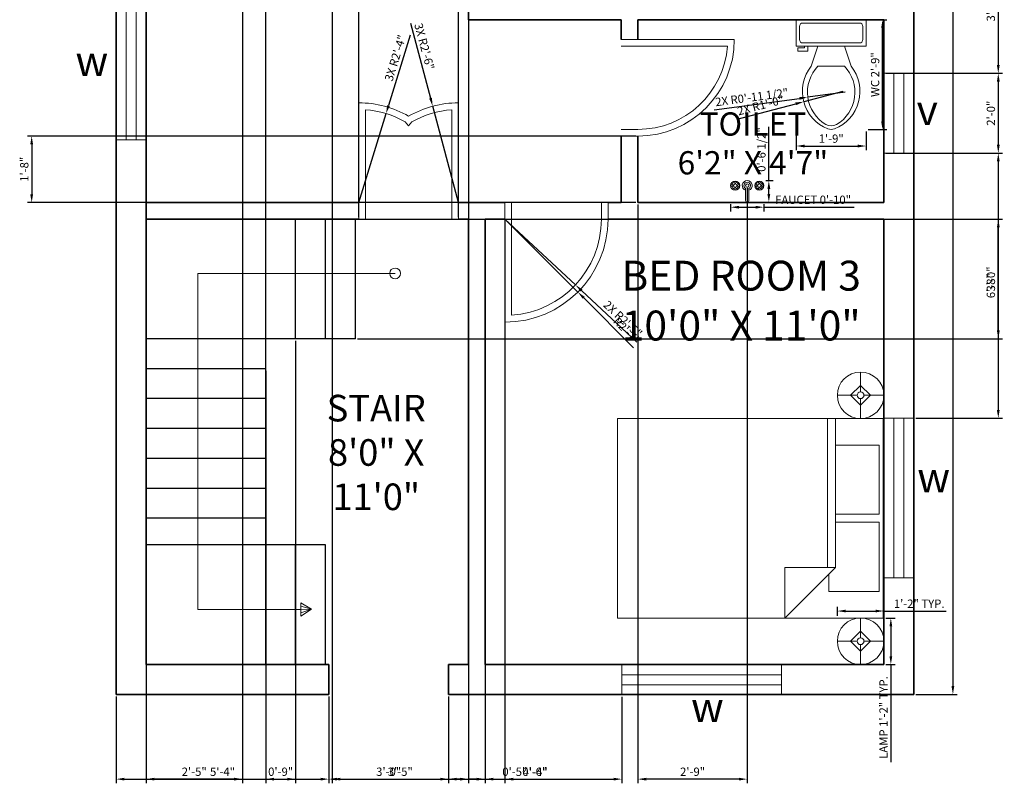
# Model space of a CAD drawing. Units: inches. Extents: x 3796 to 4094, y 4410 to 4948.
# Tile 1 of 3: x 3798 to 4094, y 4410 to 4640. Entities that reach past the tile are written whole.
import ezdxf

# ---------------------------------------------------------------- set-up
doc = ezdxf.new("R2010")
doc.units = ezdxf.units.IN
for name, color, linetype, lineweight in [('A-ANNO-DIMS', 2, 'Continuous', 18), ('A-ANNO-SYMB', 2, 'Continuous', 13), ('A-ANNO-TEXT', 7, 'Continuous', 18), ('A-AREA-IDEN', 7, 'Continuous', 25), ('A-DOOR', 3, 'Continuous', 18), ('A-FLOR-FIXT', 9, 'Continuous', 18), ('A-FLOR-STRS', 7, 'Continuous', 25), ('A-FURN', 8, 'Continuous', 18), ('A-GLAZ', 4, 'Continuous', 18), ('A-WALL', 7, 'Continuous', 35)]:
    doc.layers.add(name, color=color, linetype=linetype, lineweight=lineweight)
doc.styles.get("Standard").update_dxf_attribs({"font": 'arial.ttf'})
doc.dimstyles.new('ISO-25', dxfattribs={"dimtxt": 2.5, "dimasz": 2.5, "dimexe": 1.25, "dimexo": 0.625, "dimtad": 1, "dimdec": 0, "dimlunit": 3, "dimtxsty": 'Standard', "dimcen": 2.5, "dimadec": 0, "dimazin": 0, "dimtfac": 1, "dimtdec": 0, "dimtmove": 0, "dimatfit": 3, "dimfxl": 1, "dimarcsym": 0})

# ---------------------------------------------------------------- blocks, each defined once
blk = doc.blocks.new('*D2')
at = {"layer": 'A-ANNO-DIMS', "color": 0, "lineweight": -2, "transparency": 16777216}
for p, q in [((4067.39, 4916.55), (4079.78, 4916.55)), ((4078.53, 4914.05), (4078.53, 4439.05)), ((4067.39, 4436.55), (4079.78, 4436.55))]:
    blk.add_line(p, q, dxfattribs=at)
at = {"layer": 'A-ANNO-DIMS', "color": 0, "transparency": 16777216}
for points in [[(4078.11, 4914.05), (4078.94, 4914.05), (4078.53, 4916.55)], [(4078.11, 4439.05), (4078.94, 4439.05), (4078.53, 4436.55)]]:
    blk.add_solid(points, dxfattribs=at)
at = {"layer": 'Defpoints', "color": 0, "transparency": 16777216}
for p in [(4066.76, 4916.55), (4066.76, 4436.55), (4078.53, 4436.55)]:
    blk.add_point(p, dxfattribs=at)
at = {"layer": 'A-ANNO-DIMS', "color": 0, "transparency": 16777216, "insert": (4076.62, 4676.55), "char_height": 2.5, "attachment_point": 5, "rotation": 90}
blk.add_mtext("40'", dxfattribs=at)
blk = doc.blocks.new('Toilet - top')
for p, q in [((9.5, -6), (9.5, -2)), ((-10, -8.5), (-8, -8.5)), ((-10, -9.5), (-10, -8.5)), ((-8, -8.5), (-8, -8)), ((-7, -8), (-7, -9.5)), ((-4, -8), (-6, -14)), ((4, -8), (6, -14)), ((-7, -9.5), (-10, -9.5)), ((4, -14), (-4, -14))]:
    blk.add_line(p, q)
blk.add_lwpolyline([(10.5, -8), (10.5, 0), (-10.5, 0), (-10.5, -8)], close=True)
for points in [[(-9.5, -2), (-9.5, -6)], [(8.5, -1), (-8.5, -1)], [(-8.5, -7), (8.5, -7)]]:
    blk.add_lwpolyline(points)
for centre, radius, start, end in [((-8.62, -1.88), 0.884, 81.8699, 188.1301), ((8.62, -1.88), 0.884, 351.8699, 98.1301), ((-8.62, -6.12), 0.884, 171.8699, 278.1301), ((8.62, -6.12), 0.884, 261.8699, 8.1301), ((3.52, -21.58), 12.17, 141.4691, 247.9714), ((4.2, -21.82), 11.33, 136.3677, 238.9468), ((-3.52, -21.58), 12.17, 292.0284, 38.5307), ((-4.2, -21.82), 11.33, 301.053, 43.6321), ((0, -27.88), 4, 245.7318, 294.2682), ((0, -29), 4, 254.8605, 285.1395)]:
    blk.add_arc(centre, radius, start, end)
blk = doc.blocks.new('Faucet - Bathroom top')
for p, q in [((-4.107, 0.125), (-4.375, 0.125)), ((-3.75, 0.4788), (-3.75, 0.75)), ((-3.5, 0.482), (-3.5, 0.75)), ((-3.1461, 0.125), (-2.875, 0.125)), ((3.143, 0.125), (2.875, 0.125)), ((3.5, 0.4788), (3.5, 0.75)), ((3.75, 0.482), (3.75, 0.75)), ((4.1039, 0.125), (4.375, 0.125)), ((-4.1039, -0.125), (-4.375, -0.125)), ((-3.75, -0.4821), (-3.75, -0.75)), ((-3.5, -0.4789), (-3.5, -0.75)), ((-3.143, -0.125), (-2.875, -0.125)), ((-0.5, -0.8639), (-0.5, -4.5)), ((0.5, -4.5), (0.5, -0.8631)), ((3.1461, -0.125), (2.875, -0.125)), ((3.5, -0.4821), (3.5, -0.75)), ((3.75, -0.4789), (3.75, -0.75)), ((4.107, -0.125), (4.375, -0.125))]:
    blk.add_line(p, q)
for centre, radius in [((-3.625, 0), 1.375), ((-4.625, 0), 0.2795), ((-3.625, 0), 0.5), ((-3.625, 1), 0.2795), ((-2.625, 0), 0.2795), ((0, 0), 0.5), ((3.625, 0), 1.375), ((2.625, 0), 0.2795), ((3.625, 0), 0.5), ((3.625, 1), 0.2795), ((4.625, 0), 0.2795), ((-3.625, -1), 0.2795), ((3.625, -1), 0.2795)]:
    blk.add_circle(centre, radius)
for centre, radius, start, end in [((-3.625, 0), 1, 105.2407, 164.2093), ((-3.625, 0), 1, 16.44125, 74.07887), ((0, 0), 1.5, 289.6514, 250.3603), ((0, 0), 1, 300.3431, 239.7554), ((3.625, 0), 1, 106.12, 164.0884), ((3.625, 0), 1, 16.23422, 73.90469), ((-3.625, 0), 1, 196.2342, 253.9047), ((-3.625, 0), 1, 286.12, 344.0884), ((3.625, 0), 1, 196.4413, 254.0789), ((3.625, 0), 1, 285.2407, 344.2093), ((0, -4.5), 0.5, 180, 0)]:
    blk.add_arc(centre, radius, start, end)
blk = doc.blocks.new('Bed - Queen')
for p, q in [((0, -80.00003), (0, 0)), ((0, 0), (59.99999, 0)), ((59.99999, 0), (59.99999, -80.00003)), ((7.99999, -1.2), (28.79998, -1.2)), ((7.99999, -14.4), (7.99999, -1.2)), ((28.79998, -1.2), (28.79998, -14.4)), ((31.19999, -1.2), (51.99999, -1.2)), ((31.19999, -14.4), (31.19999, -1.2)), ((51.99999, -1.2), (51.99999, -16.4)), ((0, -14.4), (44.8, -14.4)), ((59.99999, -29.6), (44.8, -14.4)), ((44.8, -14.4), (44.8, -29.6)), ((44.8, -16.8), (0, -16.8)), ((51.99999, -16.4), (46.79936, -16.4)), ((44.8, -29.6), (59.99999, -29.6)), ((59.99999, -80.00003), (0, -80.00003))]:
    blk.add_line(p, q)
blk = doc.blocks.new('Lamp - Table')
for p, q in [((0, 7), (0, 1)), ((0, 3), (-3, 0)), ((3, 0), (0, 3)), ((-1, 0), (-7, 0)), ((-3, 0), (0, -3)), ((0, -3), (3, 0)), ((1, 0), (7, 0)), ((0, -1), (0, -7))]:
    blk.add_line(p, q)
for radius in [7, 1]:
    blk.add_circle((0, 0), radius)
blk = doc.blocks.new('WIN-48IN')
for p, q in [((0, 48), (0, 0)), ((9, 48), (0, 48)), ((3, 48), (3, 0)), ((6, 0), (6, 48)), ((9, 0), (9, 48)), ((0, 0), (9, 0))]:
    blk.add_line(p, q)
blk = doc.blocks.new('DOOR-SWING-29IN')
for p, q in [((0, 0), (-29, 0)), ((0, 0), (5, 0)), ((0, -2), (-26.93, -2)), ((0, -2), (5, -2)), ((5, -27), (0, -27)), ((5, -29), (0, -29))]:
    blk.add_line(p, q)
for radius, start in [(29, 180), (27, 184.248)]:
    blk.add_arc((0, 0), radius, start, 270)
blk = doc.blocks.new('*D17')
at = {"layer": 'A-ANNO-DIMS', "color": 0, "lineweight": -2, "transparency": 16777216}
for p, q in [((4058.39, 4459.55), (4061.11, 4459.55)), ((4059.86, 4457.05), (4059.86, 4448.05)), ((4058.39, 4445.55), (4061.11, 4445.55)), ((4059.86, 4445.55), (4059.86, 4416.19))]:
    blk.add_line(p, q, dxfattribs=at)
at = {"layer": 'A-ANNO-DIMS', "color": 0, "transparency": 16777216}
for points in [[(4059.45, 4457.05), (4060.28, 4457.05), (4059.86, 4459.55)], [(4059.45, 4448.05), (4060.28, 4448.05), (4059.86, 4445.55)]]:
    blk.add_solid(points, dxfattribs=at)
at = {"layer": 'Defpoints', "color": 0, "transparency": 16777216}
for p in [(4057.76, 4459.55), (4057.76, 4445.55), (4059.86, 4445.55)]:
    blk.add_point(p, dxfattribs=at)
at = {"layer": 'A-ANNO-DIMS', "color": 0, "transparency": 16777216, "insert": (4057.98, 4429.62), "char_height": 2.5, "attachment_point": 5, "rotation": 90}
blk.add_mtext('LAMP 1\'-2" TYP.', dxfattribs=at)
blk = doc.blocks.new('*D18')
at = {"layer": 'A-ANNO-DIMS', "color": 0, "lineweight": -2, "transparency": 16777216}
for p, q in [((4043.76, 4460.18), (4043.76, 4462.9)), ((4057.76, 4460.18), (4057.76, 4462.9)), ((4046.26, 4461.65), (4055.26, 4461.65)), ((4057.76, 4461.65), (4076.52, 4461.65))]:
    blk.add_line(p, q, dxfattribs=at)
at = {"layer": 'A-ANNO-DIMS', "color": 0, "transparency": 16777216}
for points in [[(4046.26, 4462.07), (4046.26, 4461.24), (4043.76, 4461.65)], [(4055.26, 4462.07), (4055.26, 4461.24), (4057.76, 4461.65)]]:
    blk.add_solid(points, dxfattribs=at)
at = {"layer": 'Defpoints', "color": 0, "transparency": 16777216}
for p in [(4043.76, 4459.55), (4057.76, 4461.65), (4057.76, 4459.55)]:
    blk.add_point(p, dxfattribs=at)
at = {"layer": 'A-ANNO-DIMS', "color": 0, "transparency": 16777216, "insert": (4068.39, 4463.53), "char_height": 2.5, "attachment_point": 5}
blk.add_mtext('1\'-2" TYP.', dxfattribs=at)
blk = doc.blocks.new('*D23')
at = {"layer": 'A-ANNO-DIMS', "color": 0, "lineweight": -2, "transparency": 16777216}
for p, q in [((4053.03, 4639.55), (4058.61, 4639.55)), ((4057.36, 4609.01), (4057.36, 4637.05)), ((4053.03, 4606.51), (4058.61, 4606.51))]:
    blk.add_line(p, q, dxfattribs=at)
at = {"layer": 'A-ANNO-DIMS', "color": 0, "transparency": 16777216}
for points in [[(4056.95, 4637.05), (4057.78, 4637.05), (4057.36, 4639.55)], [(4056.95, 4609.01), (4057.78, 4609.01), (4057.36, 4606.51)]]:
    blk.add_solid(points, dxfattribs=at)
at = {"layer": 'Defpoints', "color": 0, "transparency": 16777216}
for p in [(4052.41, 4639.55), (4057.36, 4639.55), (4052.41, 4606.51)]:
    blk.add_point(p, dxfattribs=at)
at = {"layer": 'A-ANNO-DIMS', "color": 0, "transparency": 16777216, "insert": (4055.45, 4623.03), "char_height": 2.5, "attachment_point": 5, "rotation": 90}
blk.add_mtext('WC 2\'-9"', dxfattribs=at)
blk = doc.blocks.new('*D24')
at = {"layer": 'A-ANNO-DIMS', "color": 0, "lineweight": -2, "transparency": 16777216}
for p, q in [((4031.41, 4605.88), (4031.41, 4600.3)), ((4052.41, 4605.88), (4052.41, 4600.3)), ((4033.91, 4601.55), (4049.91, 4601.55))]:
    blk.add_line(p, q, dxfattribs=at)
at = {"layer": 'A-ANNO-DIMS', "color": 0, "transparency": 16777216}
for points in [[(4033.91, 4601.97), (4033.91, 4601.13), (4031.41, 4601.55)], [(4049.91, 4601.97), (4049.91, 4601.13), (4052.41, 4601.55)]]:
    blk.add_solid(points, dxfattribs=at)
at = {"layer": 'Defpoints', "color": 0, "transparency": 16777216}
for p in [(4031.41, 4606.51), (4052.41, 4606.51), (4052.41, 4601.55)]:
    blk.add_point(p, dxfattribs=at)
at = {"layer": 'A-ANNO-DIMS', "color": 0, "transparency": 16777216, "insert": (4041.91, 4603.45), "char_height": 2.5, "attachment_point": 5}
blk.add_mtext('1\'-9"', dxfattribs=at)
blk = doc.blocks.new('*D25')
at = {"layer": 'A-ANNO-DIMS', "color": 0, "lineweight": -2, "transparency": 16777216}
for p, q in [((4011.65, 4584.01), (4011.65, 4581.89)), ((4021.65, 4584.01), (4021.65, 4581.89)), ((4014.15, 4583.14), (4019.15, 4583.14)), ((4021.65, 4583.14), (4048.79, 4583.14))]:
    blk.add_line(p, q, dxfattribs=at)
at = {"layer": 'A-ANNO-DIMS', "color": 0, "transparency": 16777216}
for points in [[(4014.15, 4583.55), (4014.15, 4582.72), (4011.65, 4583.14)], [(4019.15, 4583.55), (4019.15, 4582.72), (4021.65, 4583.14)]]:
    blk.add_solid(points, dxfattribs=at)
at = {"layer": 'Defpoints', "color": 0, "transparency": 16777216}
for p in [(4011.65, 4584.64), (4021.65, 4584.64), (4021.65, 4583.14)]:
    blk.add_point(p, dxfattribs=at)
at = {"layer": 'A-ANNO-DIMS', "color": 0, "transparency": 16777216, "insert": (4036.47, 4585.06), "char_height": 2.5, "attachment_point": 5}
blk.add_mtext('FAUCET 0\'-10"', dxfattribs=at)
blk = doc.blocks.new('*D26')
at = {"layer": 'A-ANNO-DIMS', "color": 0, "lineweight": -2, "transparency": 16777216}
for p, q in [((4023.15, 4591.14), (4023.15, 4607.36)), ((4022.28, 4591.14), (4024.4, 4591.14)), ((4023.15, 4587.14), (4023.15, 4588.64)), ((4022.28, 4584.64), (4024.4, 4584.64))]:
    blk.add_line(p, q, dxfattribs=at)
at = {"layer": 'A-ANNO-DIMS', "color": 0, "transparency": 16777216}
for points in [[(4022.73, 4588.64), (4023.57, 4588.64), (4023.15, 4591.14)], [(4022.73, 4587.14), (4023.57, 4587.14), (4023.15, 4584.64)]]:
    blk.add_solid(points, dxfattribs=at)
at = {"layer": 'Defpoints', "color": 0, "transparency": 16777216}
for p in [(4021.65, 4591.14), (4023.15, 4591.14), (4021.65, 4584.64)]:
    blk.add_point(p, dxfattribs=at)
at = {"layer": 'A-ANNO-DIMS', "color": 0, "transparency": 16777216, "insert": (4021.23, 4600.5), "char_height": 2.5, "attachment_point": 5, "rotation": 90}
blk.add_mtext('0\'-6 1/2"', dxfattribs=at)
blk = doc.blocks.new('*D27')
at = {"layer": 'A-ANNO-DIMS', "color": 0, "lineweight": -2, "transparency": 16777216}
for p, q in [((3826.76, 4435.93), (3826.76, 4409.83)), ((3890.76, 4435.93), (3890.76, 4409.83)), ((3829.26, 4411.08), (3888.26, 4411.08))]:
    blk.add_line(p, q, dxfattribs=at)
at = {"layer": 'A-ANNO-DIMS', "color": 0, "transparency": 16777216}
for points in [[(3829.26, 4411.49), (3829.26, 4410.66), (3826.76, 4411.08)], [(3888.26, 4411.49), (3888.26, 4410.66), (3890.76, 4411.08)]]:
    blk.add_solid(points, dxfattribs=at)
at = {"layer": 'Defpoints', "color": 0, "transparency": 16777216}
for p in [(3826.76, 4436.55), (3890.76, 4436.55), (3890.76, 4411.08)]:
    blk.add_point(p, dxfattribs=at)
at = {"layer": 'A-ANNO-DIMS', "color": 0, "transparency": 16777216, "insert": (3858.76, 4412.97), "char_height": 2.5, "attachment_point": 5}
blk.add_mtext('5\'-4"', dxfattribs=at)
blk = doc.blocks.new('*D28')
at = {"layer": 'A-ANNO-DIMS', "color": 0, "lineweight": -2, "transparency": 16777216}
for p, q in [((3890.76, 4435.93), (3890.76, 4409.83)), ((3926.76, 4435.93), (3926.76, 4409.83)), ((3893.26, 4411.08), (3924.26, 4411.08))]:
    blk.add_line(p, q, dxfattribs=at)
at = {"layer": 'A-ANNO-DIMS', "color": 0, "transparency": 16777216}
for points in [[(3893.26, 4411.49), (3893.26, 4410.66), (3890.76, 4411.08)], [(3924.26, 4411.49), (3924.26, 4410.66), (3926.76, 4411.08)]]:
    blk.add_solid(points, dxfattribs=at)
at = {"layer": 'Defpoints', "color": 0, "transparency": 16777216}
for p in [(3890.76, 4436.55), (3926.76, 4436.55), (3926.76, 4411.08)]:
    blk.add_point(p, dxfattribs=at)
at = {"layer": 'A-ANNO-DIMS', "color": 0, "transparency": 16777216, "insert": (3908.76, 4412.98), "char_height": 2.5, "attachment_point": 5}
blk.add_mtext('3\'-0"', dxfattribs=at)
blk = doc.blocks.new('*D29')
at = {"layer": 'A-ANNO-DIMS', "color": 0, "lineweight": -2, "transparency": 16777216}
for p, q in [((3926.76, 4435.93), (3926.76, 4409.83)), ((3978.92, 4435.88), (3978.92, 4409.83)), ((3929.26, 4411.08), (3976.42, 4411.08))]:
    blk.add_line(p, q, dxfattribs=at)
at = {"layer": 'A-ANNO-DIMS', "color": 0, "transparency": 16777216}
for points in [[(3929.26, 4411.49), (3929.26, 4410.66), (3926.76, 4411.08)], [(3976.42, 4411.49), (3976.42, 4410.66), (3978.92, 4411.08)]]:
    blk.add_solid(points, dxfattribs=at)
at = {"layer": 'Defpoints', "color": 0, "transparency": 16777216}
for p in [(3926.76, 4436.55), (3978.92, 4436.5), (3978.92, 4411.08)]:
    blk.add_point(p, dxfattribs=at)
at = {"layer": 'A-ANNO-DIMS', "color": 0, "transparency": 16777216, "insert": (3952.84, 4412.95), "char_height": 2.5, "attachment_point": 5}
blk.add_mtext('4\'-4"', dxfattribs=at)
blk = doc.blocks.new('*D30')
at = {"layer": 'A-ANNO-DIMS', "color": 0, "lineweight": -2, "transparency": 16777216}
for p, q in [((3932.76, 4444.93), (3932.76, 4409.83)), ((3937.76, 4444.93), (3937.76, 4409.83)), ((3930.26, 4411.08), (3927.76, 4411.08)), ((3932.76, 4411.08), (3937.76, 4411.08)), ((3940.26, 4411.08), (3950.66, 4411.08))]:
    blk.add_line(p, q, dxfattribs=at)
at = {"layer": 'A-ANNO-DIMS', "color": 0, "transparency": 16777216}
for points in [[(3930.26, 4411.49), (3930.26, 4410.66), (3932.76, 4411.08)], [(3940.26, 4411.49), (3940.26, 4410.66), (3937.76, 4411.08)]]:
    blk.add_solid(points, dxfattribs=at)
at = {"layer": 'Defpoints', "color": 0, "transparency": 16777216}
for p in [(3932.76, 4445.55), (3937.76, 4445.55), (3937.76, 4411.08)]:
    blk.add_point(p, dxfattribs=at)
at = {"layer": 'A-ANNO-DIMS', "color": 0, "transparency": 16777216, "insert": (3946.71, 4412.98), "char_height": 2.5, "attachment_point": 5}
blk.add_mtext('0\'-5"', dxfattribs=at)
blk = doc.blocks.new('*D31')
at = {"layer": 'A-ANNO-DIMS', "color": 0, "lineweight": -2, "transparency": 16777216}
for p, q in [((3835.76, 4482.18), (3835.76, 4943.23)), ((3838.26, 4941.98), (3869.26, 4941.98)), ((3871.76, 4490.18), (3871.76, 4943.23))]:
    blk.add_line(p, q, dxfattribs=at)
at = {"layer": 'A-ANNO-DIMS', "color": 0, "transparency": 16777216}
for points in [[(3838.26, 4942.39), (3838.26, 4941.56), (3835.76, 4941.98)], [(3869.26, 4942.39), (3869.26, 4941.56), (3871.76, 4941.98)]]:
    blk.add_solid(points, dxfattribs=at)
at = {"layer": 'Defpoints', "color": 0, "transparency": 16777216}
for p in [(3871.76, 4941.98), (3871.76, 4489.55), (3835.76, 4481.55)]:
    blk.add_point(p, dxfattribs=at)
at = {"layer": 'A-ANNO-DIMS', "color": 0, "transparency": 16777216, "insert": (3853.76, 4943.88), "char_height": 2.5, "attachment_point": 5}
blk.add_mtext('3\'-0"', dxfattribs=at)
blk = doc.blocks.new('*D32')
at = {"layer": 'A-ANNO-DIMS', "color": 0, "lineweight": -2, "transparency": 16777216}
for p, q in [((3880.76, 4542.93), (3880.76, 4409.83)), ((3871.76, 4533.93), (3871.76, 4409.83)), ((3874.26, 4411.08), (3878.26, 4411.08))]:
    blk.add_line(p, q, dxfattribs=at)
at = {"layer": 'A-ANNO-DIMS', "color": 0, "transparency": 16777216}
for points in [[(3874.26, 4411.49), (3874.26, 4410.66), (3871.76, 4411.08)], [(3878.26, 4411.49), (3878.26, 4410.66), (3880.76, 4411.08)]]:
    blk.add_solid(points, dxfattribs=at)
at = {"layer": 'Defpoints', "color": 0, "transparency": 16777216}
for p in [(3880.76, 4543.55), (3871.76, 4534.55), (3880.76, 4411.08)]:
    blk.add_point(p, dxfattribs=at)
at = {"layer": 'A-ANNO-DIMS', "color": 0, "transparency": 16777216, "insert": (3876.26, 4412.98), "char_height": 2.5, "attachment_point": 5}
blk.add_mtext('0\'-9"', dxfattribs=at)
blk = doc.blocks.new('*D33')
at = {"layer": 'A-ANNO-DIMS', "color": 0, "lineweight": -2, "transparency": 16777216}
for p, q in [((3899.39, 4579.55), (4093.44, 4579.55)), ((4092.19, 4546.05), (4092.19, 4577.05)), ((3899.39, 4543.55), (4093.44, 4543.55))]:
    blk.add_line(p, q, dxfattribs=at)
at = {"layer": 'A-ANNO-DIMS', "color": 0, "transparency": 16777216}
for points in [[(4091.77, 4577.05), (4092.61, 4577.05), (4092.19, 4579.55)], [(4091.77, 4546.05), (4092.61, 4546.05), (4092.19, 4543.55)]]:
    blk.add_solid(points, dxfattribs=at)
at = {"layer": 'Defpoints', "color": 0, "transparency": 16777216}
for p in [(3898.76, 4579.55), (4092.19, 4579.55), (3898.76, 4543.55)]:
    blk.add_point(p, dxfattribs=at)
at = {"layer": 'A-ANNO-DIMS', "color": 0, "transparency": 16777216, "insert": (4090.29, 4561.55), "char_height": 2.5, "attachment_point": 5, "rotation": 90}
blk.add_mtext('3\'-0"', dxfattribs=at)
blk = doc.blocks.new('*D34')
at = {"layer": 'A-ANNO-DIMS', "color": 0, "lineweight": -2, "transparency": 16777216}
for p, q in [((3899.76, 4580.18), (3899.76, 4943.23)), ((3902.26, 4941.98), (3927.26, 4941.98)), ((3929.76, 4580.18), (3929.76, 4943.23))]:
    blk.add_line(p, q, dxfattribs=at)
at = {"layer": 'A-ANNO-DIMS', "color": 0, "transparency": 16777216}
for points in [[(3902.26, 4942.39), (3902.26, 4941.56), (3899.76, 4941.98)], [(3927.26, 4942.39), (3927.26, 4941.56), (3929.76, 4941.98)]]:
    blk.add_solid(points, dxfattribs=at)
at = {"layer": 'Defpoints', "color": 0, "transparency": 16777216}
for p in [(3929.76, 4941.98), (3899.76, 4579.55), (3929.76, 4579.55)]:
    blk.add_point(p, dxfattribs=at)
at = {"layer": 'A-ANNO-DIMS', "color": 0, "transparency": 16777216, "insert": (3914.76, 4943.88), "char_height": 2.5, "attachment_point": 5}
blk.add_mtext('2\'-6"', dxfattribs=at)
blk = doc.blocks.new('*D42')
at = {"layer": 'A-ANNO-DIMS', "color": 0, "lineweight": -2, "transparency": 16777216}
for p, q in [((4067.39, 4668.03), (4093.44, 4668.03)), ((4092.19, 4665.53), (4092.19, 4625.92)), ((4067.39, 4623.42), (4093.44, 4623.42))]:
    blk.add_line(p, q, dxfattribs=at)
at = {"layer": 'A-ANNO-DIMS', "color": 0, "transparency": 16777216}
for points in [[(4091.77, 4665.53), (4092.61, 4665.53), (4092.19, 4668.03)], [(4091.77, 4625.92), (4092.61, 4625.92), (4092.19, 4623.42)]]:
    blk.add_solid(points, dxfattribs=at)
at = {"layer": 'Defpoints', "color": 0, "transparency": 16777216}
for p in [(4066.76, 4668.03), (4066.76, 4623.42), (4092.19, 4623.42)]:
    blk.add_point(p, dxfattribs=at)
at = {"layer": 'A-ANNO-DIMS', "color": 0, "transparency": 16777216, "insert": (4090.27, 4645.73), "char_height": 2.5, "attachment_point": 5, "rotation": 90}
blk.add_mtext('3\'-8 1/2"', dxfattribs=at)
blk = doc.blocks.new('*D43')
at = {"layer": 'A-ANNO-DIMS', "color": 0, "lineweight": -2, "transparency": 16777216}
for p, q in [((4058.39, 4623.42), (4093.44, 4623.42)), ((4092.19, 4620.92), (4092.19, 4601.92)), ((4058.39, 4599.42), (4093.44, 4599.42))]:
    blk.add_line(p, q, dxfattribs=at)
at = {"layer": 'A-ANNO-DIMS', "color": 0, "transparency": 16777216}
for points in [[(4091.77, 4620.92), (4092.61, 4620.92), (4092.19, 4623.42)], [(4091.77, 4601.92), (4092.61, 4601.92), (4092.19, 4599.42)]]:
    blk.add_solid(points, dxfattribs=at)
at = {"layer": 'Defpoints', "color": 0, "transparency": 16777216}
for p in [(4057.76, 4623.42), (4057.76, 4599.42), (4092.19, 4599.42)]:
    blk.add_point(p, dxfattribs=at)
at = {"layer": 'A-ANNO-DIMS', "color": 0, "transparency": 16777216, "insert": (4090.29, 4611.42), "char_height": 2.5, "attachment_point": 5, "rotation": 90}
blk.add_mtext('2\'-0"', dxfattribs=at)
blk = doc.blocks.new('*D44')
at = {"layer": 'A-ANNO-DIMS', "color": 0, "lineweight": -2, "transparency": 16777216}
for p, q in [((4067.39, 4599.42), (4093.44, 4599.42)), ((4092.19, 4596.92), (4092.19, 4522.15)), ((4067.39, 4519.65), (4093.44, 4519.65))]:
    blk.add_line(p, q, dxfattribs=at)
at = {"layer": 'A-ANNO-DIMS', "color": 0, "transparency": 16777216}
for points in [[(4091.77, 4596.92), (4092.61, 4596.92), (4092.19, 4599.42)], [(4091.77, 4522.15), (4092.61, 4522.15), (4092.19, 4519.65)]]:
    blk.add_solid(points, dxfattribs=at)
at = {"layer": 'Defpoints', "color": 0, "transparency": 16777216}
for p in [(4066.76, 4599.42), (4066.76, 4519.65), (4092.19, 4519.65)]:
    blk.add_point(p, dxfattribs=at)
at = {"layer": 'A-ANNO-DIMS', "color": 0, "transparency": 16777216, "insert": (4090.29, 4559.53), "char_height": 2.5, "attachment_point": 5, "rotation": 90}
blk.add_mtext('6\'-8"', dxfattribs=at)
blk = doc.blocks.new('*D45')
at = {"layer": 'A-ANNO-DIMS', "color": 0, "lineweight": -2, "transparency": 16777216}
for p, q in [((3835.76, 4824.93), (3835.76, 4409.83)), ((3864.76, 4824.93), (3864.76, 4409.83)), ((3862.26, 4411.08), (3838.26, 4411.08))]:
    blk.add_line(p, q, dxfattribs=at)
at = {"layer": 'A-ANNO-DIMS', "color": 0, "transparency": 16777216}
for points in [[(3838.26, 4411.49), (3838.26, 4410.66), (3835.76, 4411.08)], [(3862.26, 4411.49), (3862.26, 4410.66), (3864.76, 4411.08)]]:
    blk.add_solid(points, dxfattribs=at)
at = {"layer": 'Defpoints', "color": 0, "transparency": 16777216}
for p in [(3835.76, 4825.55), (3864.76, 4825.55), (3835.76, 4411.08)]:
    blk.add_point(p, dxfattribs=at)
at = {"layer": 'A-ANNO-DIMS', "color": 0, "transparency": 16777216, "insert": (3850.26, 4412.98), "char_height": 2.5, "attachment_point": 5}
blk.add_mtext('2\'-5"', dxfattribs=at)
blk = doc.blocks.new('*D49')
at = {"layer": 'A-ANNO-DIMS', "color": 0, "lineweight": -2, "transparency": 16777216}
for p, q in [((4016.65, 4589.01), (4016.65, 4409.83)), ((3983.76, 4583.93), (3983.76, 4409.83)), ((4014.15, 4411.08), (3986.26, 4411.08))]:
    blk.add_line(p, q, dxfattribs=at)
at = {"layer": 'A-ANNO-DIMS', "color": 0, "transparency": 16777216}
for points in [[(3986.26, 4411.49), (3986.26, 4410.66), (3983.76, 4411.08)], [(4014.15, 4411.49), (4014.15, 4410.66), (4016.65, 4411.08)]]:
    blk.add_solid(points, dxfattribs=at)
at = {"layer": 'Defpoints', "color": 0, "transparency": 16777216}
for p in [(4016.65, 4589.64), (3983.76, 4584.55), (3983.76, 4411.08)]:
    blk.add_point(p, dxfattribs=at)
at = {"layer": 'A-ANNO-DIMS', "color": 0, "transparency": 16777216, "insert": (4000.21, 4412.98), "char_height": 2.5, "attachment_point": 5}
blk.add_mtext('2\'-9"', dxfattribs=at)
blk = doc.blocks.new('*D50')
at = {"layer": 'A-ANNO-DIMS', "color": 0, "lineweight": -2, "transparency": 16777216}
for p, q in [((3983.14, 4604.55), (3800.09, 4604.55)), ((3801.34, 4602.05), (3801.34, 4587.05)), ((3983.14, 4584.55), (3800.09, 4584.55))]:
    blk.add_line(p, q, dxfattribs=at)
at = {"layer": 'A-ANNO-DIMS', "color": 0, "transparency": 16777216}
for points in [[(3800.92, 4602.05), (3801.76, 4602.05), (3801.34, 4604.55)], [(3800.92, 4587.05), (3801.76, 4587.05), (3801.34, 4584.55)]]:
    blk.add_solid(points, dxfattribs=at)
at = {"layer": 'Defpoints', "color": 0, "transparency": 16777216}
for p in [(3983.76, 4604.55), (3801.34, 4584.55), (3983.76, 4584.55)]:
    blk.add_point(p, dxfattribs=at)
at = {"layer": 'A-ANNO-DIMS', "color": 0, "transparency": 16777216, "insert": (3799.44, 4594.55), "char_height": 2.5, "attachment_point": 5, "rotation": 90}
blk.add_mtext('1\'-8"', dxfattribs=at)
blk = doc.blocks.new('*D53')
at = {"layer": 'A-ANNO-DIMS', "color": 0, "lineweight": -2, "transparency": 16777216}
for p, q in [((3937.76, 4578.93), (3937.76, 4409.83)), ((3943.76, 4578.93), (3943.76, 4409.83)), ((3935.26, 4411.08), (3932.76, 4411.08)), ((3937.76, 4411.08), (3943.76, 4411.08)), ((3946.26, 4411.08), (3956.66, 4411.08))]:
    blk.add_line(p, q, dxfattribs=at)
at = {"layer": 'A-ANNO-DIMS', "color": 0, "transparency": 16777216}
for points in [[(3935.26, 4411.49), (3935.26, 4410.66), (3937.76, 4411.08)], [(3946.26, 4411.49), (3946.26, 4410.66), (3943.76, 4411.08)]]:
    blk.add_solid(points, dxfattribs=at)
at = {"layer": 'Defpoints', "color": 0, "transparency": 16777216}
for p in [(3937.76, 4579.55), (3943.76, 4579.55), (3943.76, 4411.08)]:
    blk.add_point(p, dxfattribs=at)
at = {"layer": 'A-ANNO-DIMS', "color": 0, "transparency": 16777216, "insert": (3952.71, 4412.98), "char_height": 2.5, "attachment_point": 5}
blk.add_mtext('0\'-6"', dxfattribs=at)
blk = doc.blocks.new('*D54')
at = {"layer": 'A-ANNO-DIMS', "color": 0, "lineweight": -2, "transparency": 16777216}
for p, q in [((3891.76, 4784.93), (3891.76, 4409.83)), ((3932.76, 4786.93), (3932.76, 4409.83)), ((3894.26, 4411.08), (3930.26, 4411.08))]:
    blk.add_line(p, q, dxfattribs=at)
at = {"layer": 'A-ANNO-DIMS', "color": 0, "transparency": 16777216}
for points in [[(3894.26, 4411.49), (3894.26, 4410.66), (3891.76, 4411.08)], [(3930.26, 4411.49), (3930.26, 4410.66), (3932.76, 4411.08)]]:
    blk.add_solid(points, dxfattribs=at)
at = {"layer": 'Defpoints', "color": 0, "transparency": 16777216}
for p in [(3891.76, 4785.55), (3932.76, 4787.55), (3932.76, 4411.08)]:
    blk.add_point(p, dxfattribs=at)
at = {"layer": 'A-ANNO-DIMS', "color": 0, "transparency": 16777216, "insert": (3912.26, 4412.98), "char_height": 2.5, "attachment_point": 5}
blk.add_mtext('3\'-5"', dxfattribs=at)
blk = doc.blocks.new('*D57')
at = {"layer": 'A-ANNO-DIMS', "color": 0, "lineweight": -2, "transparency": 16777216}
for p, q in [((3943.76, 4579.55), (3965.68, 4557.63)), ((3982.47, 4540.84), (3967.45, 4555.86))]:
    blk.add_line(p, q, dxfattribs=at)
at = {"layer": 'A-ANNO-DIMS', "color": 0, "transparency": 16777216}
blk.add_solid([(3967.75, 4556.16), (3967.16, 4555.57), (3965.68, 4557.63)], dxfattribs=at)
at = {"layer": 'Defpoints', "color": 0, "transparency": 16777216}
for p in [(3943.76, 4579.55), (3965.68, 4557.63)]:
    blk.add_point(p, dxfattribs=at)
at = {"layer": 'A-ANNO-DIMS', "color": 0, "transparency": 16777216, "insert": (3980.17, 4545.81), "char_height": 2.5, "attachment_point": 5, "rotation": 314.9992}
blk.add_mtext('R2\'-7"', dxfattribs=at)
blk = doc.blocks.new('*D58')
at = {"layer": 'A-ANNO-DIMS', "color": 0, "lineweight": -2, "transparency": 16777216}
for p, q in [((3915.32, 4638.48), (3921.35, 4615.95)), ((3929.76, 4584.55), (3922, 4613.53))]:
    blk.add_line(p, q, dxfattribs=at)
at = {"layer": 'A-ANNO-DIMS', "color": 0, "transparency": 16777216}
blk.add_solid([(3921.76, 4616.05), (3920.95, 4615.84), (3922, 4613.53)], dxfattribs=at)
at = {"layer": 'Defpoints', "color": 0, "transparency": 16777216}
for p in [(3922, 4613.53), (3929.76, 4584.55)]:
    blk.add_point(p, dxfattribs=at)
at = {"layer": 'A-ANNO-DIMS', "color": 0, "transparency": 16777216, "insert": (3919.18, 4631.41), "char_height": 2.5, "attachment_point": 5, "rotation": 284.9993}
blk.add_mtext('3X R2\'-6"', dxfattribs=at)
blk = doc.blocks.new('*D59')
at = {"layer": 'A-ANNO-DIMS', "color": 0, "lineweight": -2, "transparency": 16777216}
for p, q in [((3943.76, 4579.55), (3964.97, 4559.77)), ((3983.43, 4542.54), (3966.79, 4558.06))]:
    blk.add_line(p, q, dxfattribs=at)
at = {"layer": 'A-ANNO-DIMS', "color": 0, "transparency": 16777216}
blk.add_solid([(3967.08, 4558.37), (3966.51, 4557.76), (3964.97, 4559.77)], dxfattribs=at)
at = {"layer": 'Defpoints', "color": 0, "transparency": 16777216}
for p in [(3943.76, 4579.55), (3964.97, 4559.77)]:
    blk.add_point(p, dxfattribs=at)
at = {"layer": 'A-ANNO-DIMS', "color": 0, "transparency": 16777216, "insert": (3978.98, 4549.28), "char_height": 2.5, "attachment_point": 5, "rotation": 316.9778}
blk.add_mtext('2X R2\'-5"', dxfattribs=at)
blk = doc.blocks.new('*D60')
at = {"layer": 'A-ANNO-DIMS', "color": 0, "lineweight": -2, "transparency": 16777216}
for p, q in [((3915.19, 4634.87), (3908.71, 4613.71)), ((3899.76, 4584.55), (3907.97, 4611.32))]:
    blk.add_line(p, q, dxfattribs=at)
at = {"layer": 'A-ANNO-DIMS', "color": 0, "transparency": 16777216}
blk.add_solid([(3908.31, 4613.83), (3909.1, 4613.59), (3907.97, 4611.32)], dxfattribs=at)
at = {"layer": 'Defpoints', "color": 0, "transparency": 16777216}
for p in [(3907.97, 4611.32), (3899.76, 4584.55)]:
    blk.add_point(p, dxfattribs=at)
at = {"layer": 'A-ANNO-DIMS', "color": 0, "transparency": 16777216, "insert": (3911.08, 4627.94), "char_height": 2.5, "attachment_point": 5, "rotation": 72.9519}
blk.add_mtext('3X R2\'-4"', dxfattribs=at)
blk = doc.blocks.new('*D62')
at = {"layer": 'A-ANNO-DIMS', "color": 0, "lineweight": -2, "transparency": 16777216}
for p, q in [((4045.43, 4617.97), (4033.66, 4614.88)), ((4013.63, 4609.62), (4031.24, 4614.24))]:
    blk.add_line(p, q, dxfattribs=at)
at = {"layer": 'A-ANNO-DIMS', "color": 0, "transparency": 16777216}
blk.add_solid([(4031.13, 4614.65), (4031.35, 4613.84), (4033.66, 4614.88)], dxfattribs=at)
at = {"layer": 'Defpoints', "color": 0, "transparency": 16777216}
for p in [(4045.43, 4617.97), (4033.66, 4614.88)]:
    blk.add_point(p, dxfattribs=at)
at = {"layer": 'A-ANNO-DIMS', "color": 0, "transparency": 16777216, "insert": (4020.75, 4613.45), "char_height": 2.5, "attachment_point": 5, "rotation": 14.7193}
blk.add_mtext('2X R1\'-0"', dxfattribs=at)
blk = doc.blocks.new('*D63')
at = {"layer": 'A-ANNO-DIMS', "color": 0, "lineweight": -2, "transparency": 16777216}
for p, q in [((4006.66, 4612.43), (4032.4, 4615.89)), ((4046.11, 4617.74), (4034.88, 4616.22))]:
    blk.add_line(p, q, dxfattribs=at)
at = {"layer": 'A-ANNO-DIMS', "color": 0, "transparency": 16777216}
blk.add_solid([(4032.35, 4616.3), (4032.46, 4615.48), (4034.88, 4616.22)], dxfattribs=at)
at = {"layer": 'Defpoints', "color": 0, "transparency": 16777216}
for p in [(4034.88, 4616.22), (4046.11, 4617.74)]:
    blk.add_point(p, dxfattribs=at)
at = {"layer": 'A-ANNO-DIMS', "color": 0, "transparency": 16777216, "insert": (4018.04, 4615.89), "char_height": 2.5, "attachment_point": 5, "rotation": 7.6596}
blk.add_mtext('2X R0\'-11 1/2"', dxfattribs=at)

msp = doc.modelspace()

# ---------------------------------------------------------------- linework, layer by layer
at = {"layer": 'A-ANNO-SYMB'}
for p, q in [((3910.7, 4563.23), (3851.36, 4563.23)), ((3851.36, 4563.23), (3851.36, 4462.14)), ((3851.36, 4462.14), (3882.29, 4462.14)), ((3882.29, 4462.14), (3882.29, 4464.14)), ((3882.29, 4464.14), (3885.51, 4462.23)), ((3885.51, 4462.23), (3882.29, 4463.14)), ((3882.29, 4463.14), (3885.51, 4462.23)), ((3885.51, 4462.23), (3882.29, 4460.14)), ((3882.29, 4462.14), (3885.51, 4462.23)), ((3885.51, 4462.23), (3882.29, 4461.14)), ((3882.29, 4462.14), (3882.29, 4460.14)), ((3882.29, 4460.14), (3882.29, 4462.14)), ((3882.29, 4460.14), (3882.29, 4462.14))]:
    msp.add_line(p, q, dxfattribs=at)
msp.add_circle((3910.7, 4563.23), 1.62, dxfattribs=at)
at = {"layer": 'A-DOOR'}
for p, q in [((3899.76, 4584.55), (3899.76, 4614.55)), ((3927.76, 4614.49), (3927.76, 4614.55)), ((3929.76, 4584.55), (3929.76, 4614.55)), ((3901.76, 4584.55), (3901.76, 4612.48)), ((3927.76, 4584.55), (3927.76, 4612.48)), ((3914.76, 4607.64), (3913.76, 4608.8)), ((3915.76, 4608.8), (3914.76, 4607.64)), ((3899.76, 4584.55), (3899.76, 4579.55)), ((3901.76, 4584.55), (3901.76, 4579.55)), ((3927.76, 4579.55), (3927.76, 4584.55)), ((3929.76, 4579.55), (3929.76, 4584.55)), ((3943.76, 4579.55), (3943.76, 4584.55)), ((3945.76, 4579.55), (3945.76, 4584.55)), ((3972.76, 4584.55), (3972.76, 4579.55)), ((3974.76, 4584.55), (3974.76, 4579.55)), ((3943.76, 4579.55), (3943.76, 4548.55)), ((3945.76, 4579.55), (3945.76, 4550.62))]:
    msp.add_line(p, q, dxfattribs=at)
for centre, radius, start, end in [((3899.76, 4584.55), 30, 60, 90), ((3929.76, 4584.55), 30, 90, 120), ((3899.76, 4584.55), 28, 60, 85.904), ((3929.76, 4584.55), 28, 94.096, 120), ((3943.76, 4579.55), 31, 270, 0), ((3943.76, 4579.55), 29, 273.9546, 0)]:
    msp.add_arc(centre, radius, start, end, dxfattribs=at)
at = {"layer": 'A-FLOR-STRS'}
for p, q in [((3871.76, 4445.55), (3871.76, 4579.55)), ((3880.76, 4543.55), (3880.76, 4579.55)), ((3889.76, 4543.55), (3889.76, 4579.55)), ((3898.76, 4543.55), (3898.76, 4579.55)), ((3898.76, 4543.55), (3835.76, 4543.55)), ((3871.76, 4534.55), (3835.76, 4534.55)), ((3871.76, 4525.55), (3835.76, 4525.55)), ((3871.76, 4516.55), (3835.76, 4516.55)), ((3871.76, 4507.55), (3835.76, 4507.55)), ((3871.76, 4498.55), (3835.76, 4498.55)), ((3871.76, 4489.55), (3835.76, 4489.55)), ((3889.76, 4481.55), (3835.76, 4481.55)), ((3880.76, 4445.55), (3880.76, 4481.55)), ((3889.76, 4445.55), (3889.76, 4481.55))]:
    msp.add_line(p, q, dxfattribs=at)
at = {"layer": 'A-GLAZ'}
for p, q in [((4057.76, 4623.42), (4057.76, 4599.42)), ((4066.76, 4623.42), (4057.76, 4623.42)), ((4060.76, 4623.42), (4060.76, 4599.42)), ((4063.76, 4599.42), (4063.76, 4623.42)), ((4066.76, 4599.42), (4066.76, 4623.42)), ((4057.76, 4599.42), (4066.76, 4599.42))]:
    msp.add_line(p, q, dxfattribs=at)
at = {"layer": 'A-WALL'}
for p, q in [((3826.76, 4436.55), (3826.76, 4916.55)), ((4066.76, 4916.55), (4066.76, 4436.55)), ((3835.76, 4584.55), (3835.76, 4742.55)), ((3932.76, 4734.55), (3932.76, 4639.55)), ((3932.76, 4639.55), (3978.76, 4639.55)), ((3978.76, 4639.55), (3978.76, 4633.55)), ((3983.76, 4639.55), (3983.76, 4633.55)), ((3983.76, 4639.55), (4057.76, 4639.55)), ((3983.76, 4639.55), (3983.76, 4633.55)), ((4057.76, 4639.55), (4057.76, 4584.55)), ((3978.76, 4604.55), (3978.76, 4584.55)), ((3983.76, 4604.55), (3983.76, 4584.55)), ((3899.76, 4584.55), (3835.76, 4584.55)), ((3932.76, 4584.55), (3929.76, 4584.55)), ((3932.76, 4584.55), (3943.76, 4584.55)), ((3974.76, 4584.55), (3978.76, 4584.55)), ((3983.76, 4584.55), (4057.76, 4584.55)), ((3835.76, 4445.55), (3835.76, 4579.55)), ((3899.76, 4579.55), (3835.76, 4579.55)), ((3932.76, 4579.55), (3929.76, 4579.55)), ((3932.76, 4579.55), (3929.76, 4579.55)), ((3932.76, 4579.55), (3932.76, 4445.55)), ((3937.76, 4579.55), (3943.76, 4579.55)), ((3937.76, 4579.55), (3937.76, 4445.55)), ((3937.76, 4445.55), (3937.76, 4579.55)), ((3937.76, 4579.55), (3943.76, 4579.55)), ((3974.76, 4579.55), (4057.76, 4579.55)), ((4057.76, 4579.55), (4057.76, 4445.55)), ((3890.76, 4445.55), (3835.76, 4445.55)), ((3890.76, 4436.55), (3890.76, 4445.55)), ((3932.76, 4445.55), (3926.76, 4445.55)), ((3932.76, 4445.55), (3926.76, 4445.55)), ((3926.76, 4445.55), (3926.76, 4436.55)), ((4057.76, 4445.55), (3937.76, 4445.55)), ((3890.76, 4436.55), (3826.76, 4436.55)), ((4066.76, 4436.55), (3926.76, 4436.55))]:
    msp.add_line(p, q, dxfattribs=at)

# ---------------------------------------------------------------- block references
at = {"layer": 'A-DOOR', "extrusion": (0, 0, -1), "zscale": -1}
msp.add_blockref('DOOR-SWING-29IN', (-3983.76, 4633.55), dxfattribs=at)
at = {"layer": 'A-FLOR-FIXT'}
for name, p in [('Toilet - top', (4041.91, 4639.55)), ('Faucet - Bathroom top', (4016.65, 4589.64))]:
    msp.add_blockref(name, p, dxfattribs=at)
at = {"layer": 'A-FURN', "rotation": 270}
for name, p in [('Lamp - Table', (4050.76, 4526.55)), ('Bed - Queen', (4057.58, 4519.55)), ('Lamp - Table', (4050.76, 4452.55))]:
    msp.add_blockref(name, p, dxfattribs=at)
at = {"layer": 'A-GLAZ'}
for p, rotation in [((3835.76, 4651.39), 180), ((4066.76, 4519.65), 180), ((4026.92, 4436.5), 90.00000000000315)]:
    msp.add_blockref('WIN-48IN', p, dxfattribs=dict(at, rotation=rotation))

# ---------------------------------------------------------------- texts
at = {"layer": 'A-ANNO-TEXT', "char_height": 9, "attachment_point": 1}
for s, insert in [('\\pxqc;w', (3789.97, 4631.64)), ('\\pxqc;v', (4041.34, 4616.91)), ('\\pxqc;w', (4043.27, 4506.39)), ('\\pxqc;w', (3975.18, 4437.26))]:
    msp.add_mtext_dynamic_manual_height_columns(s, width=58.9432, gutter_width=12.5, heights=[0], dxfattribs=dict(at, insert=insert))
at = {"layer": 'A-AREA-IDEN', "attachment_point": 1}
for s, width, insert, char_height in [('\\pxqc;TOILET\\P6\'2" X 4\'7"', 49.8486, (3993.44, 4611.67), 7), ('\\pxqc;BED ROOM 3\\P10\'0" X 11\'0"', 83.2593, (3973.2, 4567.04), 9), ('\\pxqc;STAIR\\P8\'0" X 11\'0"', 55.509, (3877.26, 4526.69), 8)]:
    msp.add_mtext_dynamic_manual_height_columns(s, width=width, gutter_width=12.5, heights=[0], dxfattribs=dict(at, insert=insert, char_height=char_height))

# ---------------------------------------------------------------- dimensions: what is measured, and where the dimension line sits
at = {"layer": 'A-ANNO-DIMS'}
for base, p1, p2, picture, middle in [((3871.76, 4941.98), (3835.76, 4481.55), (3871.76, 4489.55), '*D31', (3853.76, 4943.88)), ((3929.76, 4941.98), (3899.76, 4579.55), (3929.76, 4579.55), '*D34', (3914.76, 4943.88)), ((3835.76, 4411.08), (3864.76, 4825.55), (3835.76, 4825.55), '*D45', (3850.26, 4412.98)), ((3932.76, 4411.08), (3891.76, 4785.55), (3932.76, 4787.55), '*D54', (3912.26, 4412.98)), ((4052.41, 4601.55), (4031.41, 4606.51), (4052.41, 4606.51), '*D24', (4041.91, 4603.45)), ((3983.76, 4411.08), (4016.65, 4589.64), (3983.76, 4584.55), '*D49', (4000.21, 4412.98)), ((3943.76, 4411.08), (3937.76, 4579.55), (3943.76, 4579.55), '*D53', (3952.71, 4412.98)), ((3880.76, 4411.08), (3871.76, 4534.55), (3880.76, 4543.55), '*D32', (3876.26, 4412.98)), ((3937.76, 4411.08), (3932.76, 4445.55), (3937.76, 4445.55), '*D30', (3946.71, 4412.98)), ((3890.76, 4411.08), (3826.76, 4436.55), (3890.76, 4436.55), '*D27', (3858.76, 4412.97)), ((3926.76, 4411.08), (3890.76, 4436.55), (3926.76, 4436.55), '*D28', (3908.76, 4412.98)), ((3978.92, 4411.08), (3926.76, 4436.55), (3978.92, 4436.5), '*D29', (3952.84, 4412.95))]:
    dim = msp.add_linear_dim(base=base, p1=p1, p2=p2, dimstyle='ISO-25', override={"dimdec": 1, "dimlfac": 1, "dimrnd": 0, "dimzin": 1, "dimdsep": 46, "dimlunit": 4, "dimfrac": 2}, dxfattribs=at)
    dim.commit()
    dim.dimension.update_dxf_attribs({"geometry": picture, "text_midpoint": middle})
for base, p1, p2, override, picture, middle in [((4078.53, 4436.55), (4066.76, 4916.55), (4066.76, 4436.55), {"dimclrd": 0, "dimclre": 0, "dimclrt": 0}, '*D2', (4076.62, 4676.55)), ((4092.19, 4623.42), (4066.76, 4668.03), (4066.76, 4623.42), {"dimdec": 1, "dimlfac": 1, "dimrnd": 0, "dimzin": 1, "dimdsep": 46, "dimlunit": 4, "dimfrac": 2}, '*D42', (4090.27, 4645.73)), ((4092.19, 4599.42), (4057.76, 4623.42), (4057.76, 4599.42), {"dimdec": 1, "dimlfac": 1, "dimrnd": 0, "dimzin": 1, "dimdsep": 46, "dimlunit": 4, "dimfrac": 2}, '*D43', (4090.29, 4611.42)), ((4023.15, 4591.14), (4021.65, 4584.64), (4021.65, 4591.14), {"dimdec": 1, "dimlfac": 1, "dimrnd": 0, "dimzin": 1, "dimdsep": 46, "dimlunit": 4, "dimfrac": 2}, '*D26', (4021.23, 4600.5)), ((3801.34, 4584.55), (3983.76, 4604.55), (3983.76, 4584.55), {"dimdec": 1, "dimlfac": 1, "dimrnd": 0, "dimzin": 1, "dimdsep": 46, "dimlunit": 4, "dimfrac": 2}, '*D50', (3799.44, 4594.55)), ((4092.19, 4519.65), (4066.76, 4599.42), (4066.76, 4519.65), {"dimdec": 1, "dimlfac": 1, "dimrnd": 0, "dimzin": 1, "dimdsep": 46, "dimlunit": 4, "dimfrac": 2}, '*D44', (4090.29, 4559.53)), ((4092.19, 4579.55), (3898.76, 4543.55), (3898.76, 4579.55), {"dimdec": 1, "dimlfac": 1, "dimrnd": 0, "dimzin": 1, "dimdsep": 46, "dimlunit": 4, "dimfrac": 2}, '*D33', (4090.29, 4561.55))]:
    dim = msp.add_linear_dim(base=base, p1=p1, p2=p2, angle=90, dimstyle='ISO-25', override=override, dxfattribs=at)
    dim.commit()
    dim.dimension.update_dxf_attribs({"geometry": picture, "text_midpoint": middle})
for base, p1, p2, angle, text, picture, middle in [((4057.36, 4639.55), (4052.41, 4606.51), (4052.41, 4639.55), 90, 'WC <>', '*D23', (4055.45, 4623.03)), ((4059.86, 4445.55), (4057.76, 4459.55), (4057.76, 4445.55), 270, 'LAMP <> TYP.', '*D17', (4057.98, 4429.62))]:
    dim = msp.add_linear_dim(base=base, p1=p1, p2=p2, angle=angle, text=text, dimstyle='ISO-25', override={"dimdec": 1, "dimlfac": 1, "dimrnd": 0, "dimzin": 1, "dimdsep": 46, "dimlunit": 4, "dimfrac": 2}, dxfattribs=at)
    dim.commit()
    dim.dimension.update_dxf_attribs({"geometry": picture, "text_midpoint": middle})
for center, mpoint, text, picture, middle in [((3929.76, 4584.55), (3922, 4613.53), '3X <>', '*D58', (3917.34, 4630.92)), ((3899.76, 4584.55), (3907.97, 4611.32), '3X <>', '*D60', (3912.9, 4627.38)), ((3943.76, 4579.55), (3964.97, 4559.77), '2X <>', '*D59', (3977.69, 4547.89))]:
    dim = msp.add_radius_dim(center=center, mpoint=mpoint, text=text, dimstyle='ISO-25', override={"dimdec": 1, "dimlfac": 1, "dimrnd": 0, "dimzin": 1, "dimdsep": 46, "dimlunit": 4, "dimfrac": 2}, dxfattribs=at)
    dim.commit()
    dim.dimension.update_dxf_attribs({"geometry": picture, "text_midpoint": middle, "dimtype": 164})
for center, mpoint, picture, middle in [((4046.11, 4617.74), (4034.88, 4616.22), '*D63', (4018.04, 4615.89)), ((4045.43, 4617.97), (4033.66, 4614.88), '*D62', (4020.75, 4613.45))]:
    dim = msp.add_radius_dim(center=center, mpoint=mpoint, text='2X <>', dimstyle='ISO-25', override={"dimdec": 1, "dimlfac": 1, "dimrnd": 0, "dimzin": 1, "dimdsep": 46, "dimlunit": 4, "dimfrac": 2}, dxfattribs=at)
    dim.commit()
    dim.dimension.update_dxf_attribs({"geometry": picture, "text_midpoint": middle})
for base, p1, p2, text, picture, middle in [((4021.65, 4583.14), (4011.65, 4584.64), (4021.65, 4584.64), 'FAUCET <>', '*D25', (4036.47, 4585.06)), ((4057.76, 4461.65), (4043.76, 4459.55), (4057.76, 4459.55), '<> TYP.', '*D18', (4068.39, 4463.53))]:
    dim = msp.add_linear_dim(base=base, p1=p1, p2=p2, text=text, dimstyle='ISO-25', override={"dimdec": 1, "dimlfac": 1, "dimrnd": 0, "dimzin": 1, "dimdsep": 46, "dimlunit": 4, "dimfrac": 2}, dxfattribs=at)
    dim.commit()
    dim.dimension.update_dxf_attribs({"geometry": picture, "text_midpoint": middle})
dim = msp.add_radius_dim(center=(3943.76, 4579.55), mpoint=(3965.68, 4557.63), dimstyle='ISO-25', override={"dimdec": 1, "dimlfac": 1, "dimrnd": 0, "dimzin": 1, "dimdsep": 46, "dimlunit": 4, "dimfrac": 2}, dxfattribs=at)
dim.commit()
dim.dimension.update_dxf_attribs({"geometry": '*D57', "text_midpoint": (3978.84, 4544.48), "dimtype": 164})

doc.saveas('drawing.dxf')
